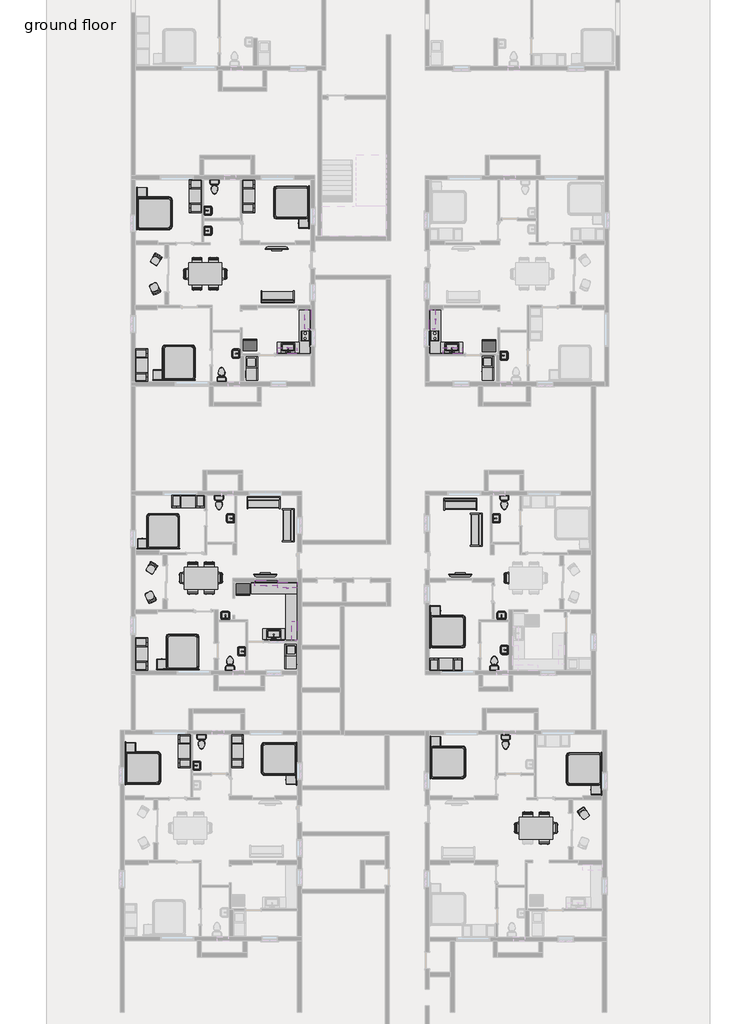
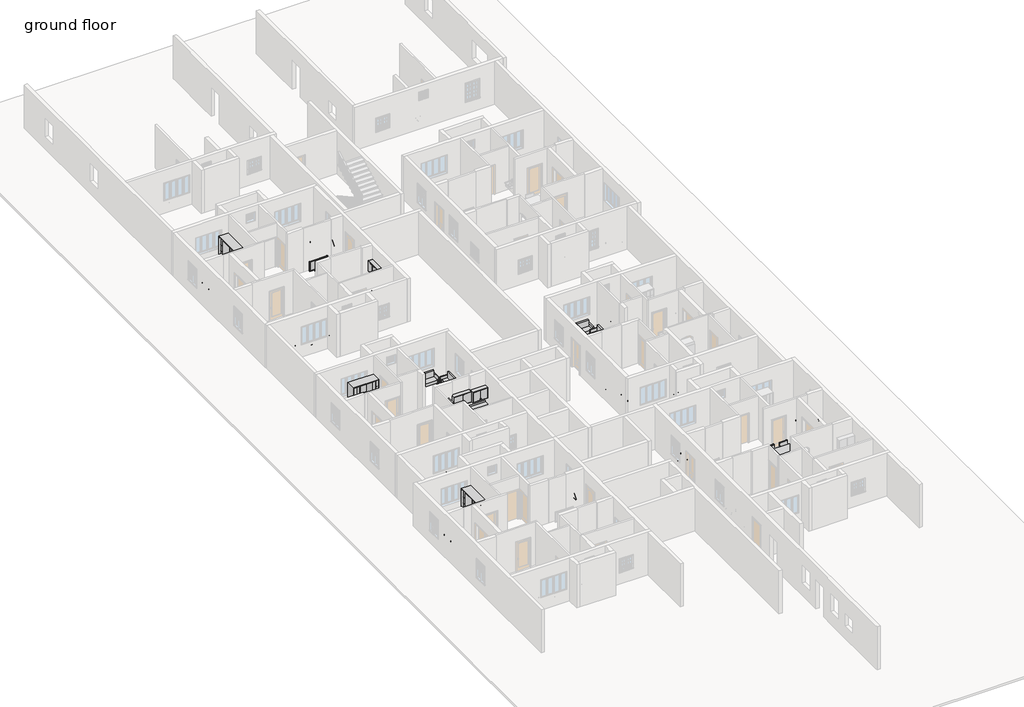
# One storey, part 12 of 16: 77 furniture elements, 22 flow terminals, 11 proxies.
# Revit data of these elements (continued)
# Elements 34, 35, 36, 37, 38, 39, 40, 41, 42, 43 (IfcFurniture, "BED_DESIGN_8999 : BED_DESIGN_8999") (continued)
#   Materials on its faces: "wood 2", "ss", "new wood", "fabric 2", "wood light", "fabric"
# Elements 44, 45, 46, 47, 48 (IfcFurniture, "Base Cabinet-Combo01 : 30\"")
#   Phase Created = New Construction
#   Materials on its faces: "Cabinet"
# Element 49 (IfcFurniture, "Base Cabinet-Combo01 : 30\" 3")
#   Phase Created = New Construction
#   Materials on its faces: "Cabinet"
# Element 50 (IfcFurniture, "Base Cabinet-Combo01 : 30\" 4")
#   Phase Created = New Construction
#   Materials on its faces: "Cabinet"
# Elements 51, 52, 53, 54 (IfcFurniture, "Base Cabinet-Corner Unit-Square : 36\"")
#   Phase Created = New Construction
#   Materials on its faces: "Cabinets", "Cabinets - Handles"
# Elements 55, 56, 57, 58, 59, 60, 61, 62, 63, 64, 65 (IfcFurniture, "Chair-Task : Chair-Task")
#   Phase Created = New Construction
#   Materials on its faces: "Plastic - Black", "Textile - Slate Blue"
# Elements 66, 67, 68, 69, 70, 71, 72 (IfcFurniture, "Chair-Task Arms : Chair-Task Arms")
#   Phase Created = New Construction
#   Materials on its faces: "Plastic - Black", "Textile - Slate Blue"
# Elements 73, 74 (IfcFurniture, "Counter Top : 24\" Depth")
#   Length = 8' - 0"
#   Phase Created = New Construction
#   Materials on its faces: "Counter Top"
# Element 75 (IfcFurniture, "Counter Top : 24\" Depth")
#   Length = 8' - 5"
#   Phase Created = New Construction
#   Materials on its faces: "Counter Top"
# Element 76 (IfcFurniture, "Counter Top : 24\" Depth")
#   Length = 8' - 4.66821"
#   Phase Created = New Construction
#   Materials on its faces: "Counter Top"
# Elements 77, 78, 79 (IfcFurniture, "Counter Top w Sink Hole : 24\" Depth")
#   Sink Opening Width = 2' - 3"
#   Sink Opening Depth = 1' - 3"
#   Sink Location To Wall = 0' - 6"
#   Sink Location = 2' - 0"
#   Length = 3' - 11.25715"
#   Phase Created = New Construction
#   Materials on its faces: "Counter Top"
# Elements 80, 81, 82, 83, 84, 85, 86, 87 (IfcFurniture, "Entertainment Center : 72\" x 72\" x 24\"")
#   Phase Created = New Construction
#   Materials on its faces: "Steel, Chrome Plated", "Glass - Clear, Grey"
# Elements 88, 89, 90, 91, 92 (IfcFurniture, "Seating-Auditorium : 18\" x 24\" x 30\"")
#   Phase Created = New Construction
#   Materials on its faces: "Steel, Paint Finish, Dark Gray, Matte", "Linen, Beige"
# Elements 93, 94, 95, 96, 97 (IfcFurniture, "Sofa : 72\"")
#   Phase Created = New Construction
#   Materials on its faces: "Cherry", "Linen, Beige"
# Elements 98, 99, 100 (IfcFurniture, "TV - Flat Screen : 50\"")
#   Stand = yes
#   Phase Created = New Construction
#   Materials on its faces: "TV - Black", "TV - Glass", "TV - Screen"
# Elements 101, 102, 103 (IfcFurniture, "Table-Conference2 w Chairs : 48\" x 144\"")
#   Phase Created = New Construction
#   Materials on its faces: "Wood - Cherry"
# Elements 104, 105, 106, 107, 108, 109 (IfcFurniture, "Upper Cabinet-Double Door-Wall : 42\"")
#   Phase Created = New Construction
#   Materials on its faces: "Cabinets - Handles", "Cabinet"
# Element 110 (IfcFurniture, "Upper Cabinet-Double Door-Wall : 42\" 2")
#   Phase Created = New Construction
#   Materials on its faces: "Cabinets - Handles", "Cabinet"
# Materials
#   "Metal - Chrome": colour RGB 57 57 57, transparency 0
#   "Metal - Steel, Polished": colour RGB 57 57 57, transparency 0
#   "Metal - Paint Finish - Ivory,Glossy": colour RGB 247 247 239, transparency 0
#   "Metal - Paint Finish - Ivory,Matte": colour RGB 247 247 239, transparency 0
#   "Steel, Polished": class "Metal", colour RGB 192 192 192, transparency 0, Description = "Polished steel", Cost = 0
#   "Porcelain, Linen": class "Ceramic", colour RGB 249 239 230, transparency 0, Description = "Porcelain, linen", Cost = 0
#   "Laminate, Linen, Matte": class "Plastic", colour RGB 249 239 230, transparency 0, Description = "Plastic Laminate - Linen, Matte", Cost = 0
#   "Cabinets": colour RGB 249 249 249, transparency 0
#   "Cabinets - Handles": colour RGB 57 57 57, transparency 0
#   "Plastic - Black": colour RGB 0 0 0, transparency 0.7
#   "Textile - Slate Blue": colour RGB 98 102 118, transparency 0
#   "Linen, Beige": class "Textile", colour RGB 249 239 230, transparency 0, Description = "Linen, beige", Cost = 0
#   "Steel, Paint Finish, Dark Gray, Matte": class "Metal", colour RGB 0 0 0, transparency 0, Description = "Steel, paint finish, dark gray, matte", Cost = 0
#   "Cherry": class "Wood", colour RGB 226 177 128, transparency 0, Description = "Prunus Serotina", Cost = 0
#   "Wood - Cherry": colour RGB 151 75 0, transparency 0
#   "wood 2": class "Wood", colour RGB 196 146 67, transparency 0
#   "ss": class "Metal", colour RGB 189 187 185, transparency 0
#   "new wood": class "Wood", colour RGB 133 62 31, transparency 0
#   "fabric 2": class "Fabric", colour RGB 198 193 133, transparency 0
#   "wood light": class "Wood", colour RGB 198 165 122, transparency 0
#   "fabric": class "Fabric", colour RGB 198 193 133, transparency 0
#   "Cabinet": colour RGB 204 122 2, transparency 0
#   "Counter Top": class "Wood", colour RGB 226 177 128, transparency 0
#   "Steel, Chrome Plated": class "Metal", colour RGB 17 17 17, transparency 0, Description = "Chromiuim plated steel", Cost = 0
#   "Glass - Clear, Grey": class "Glass", colour RGB 252 255 255, transparency 0.64
#   "TV - Black": colour RGB 49 49 49, transparency 0
#   "TV - Glass": colour RGB 157 157 157, transparency 0.9
#   "TV - Screen": colour RGB 0 0 0, transparency 0
